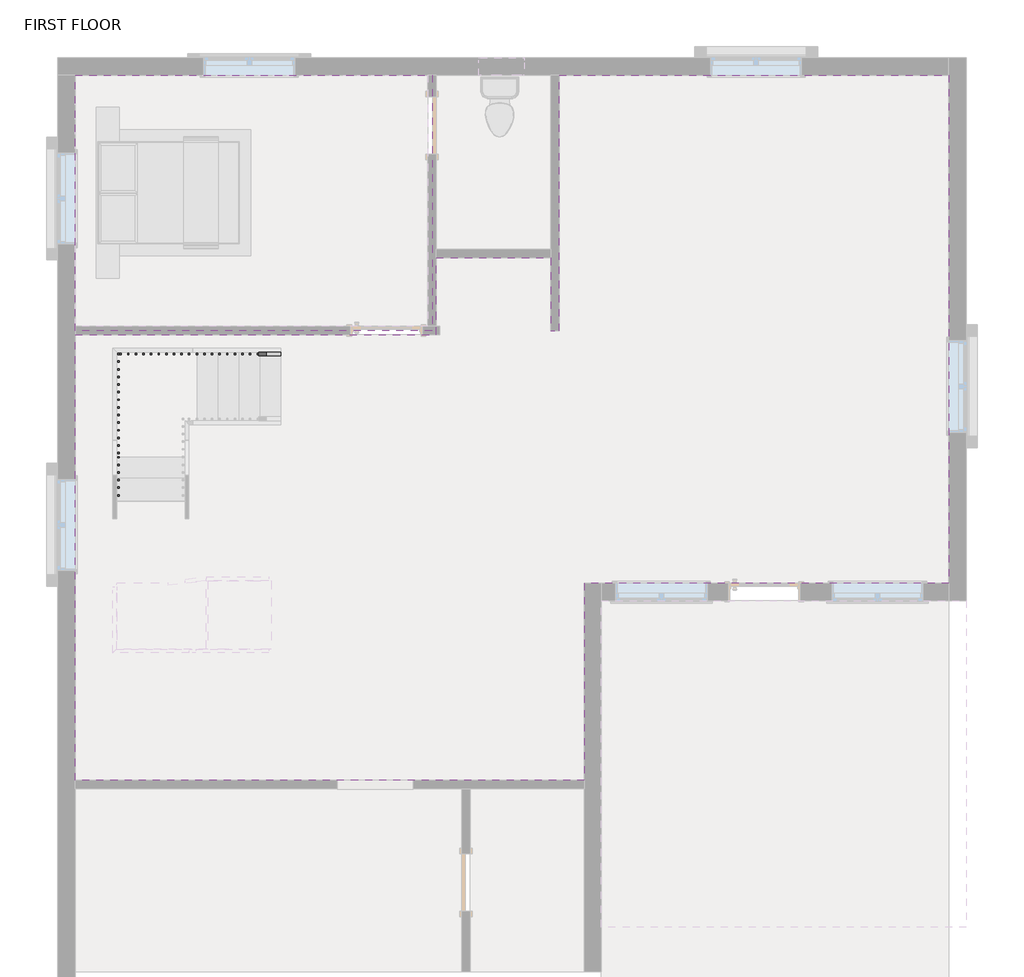
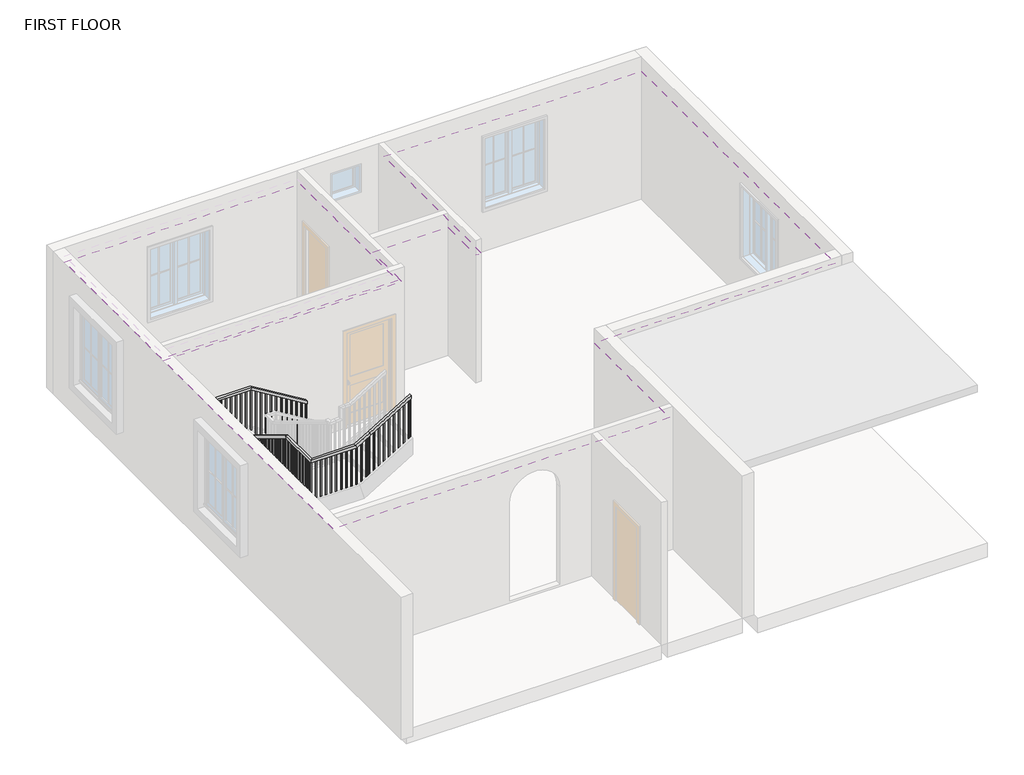
# One storey, part 2 of 4: 2 coverings, 1 railing.
"""IFC4 building model written with IfcOpenShell, lengths in millimetres."""

from ifc_helpers import new_model, si_unit, frame, origin, place, context, project, spatial, polyline, outline, extrude, faceted_brep, element, save

model = new_model("IFC4")

# Units and contexts
model_context = context("Model", 3, world=origin())
ifc_project = project(units=[si_unit("LENGTHUNIT", "METRE", prefix="MILLI")], contexts=[model_context])

# Site, building, storey
site = spatial("IfcSite", under=ifc_project)
building = spatial("IfcBuilding", under=site)
storey = spatial("IfcBuildingStorey", under=building, Name="FIRST FLOOR", Elevation=3352.8)

# Coverings
placement = place(None, origin())
element("IfcCovering", 1, ObjectType="WHITE CEILING", at=placement, inside=storey, context=model_context, shape_type="SweptSolid", body=[
    extrude(outline(polyline([(-7058.5586008, 4742.0155883), (-7058.5586008, 1332.0655883), (-11821.0586008, 1332.0655883), (-11821.0586008, 4742.0155883), (-7058.5586008, 4742.0155883)]), holes=[polyline([(-7363.3586008, 4437.2155883), (-11516.2586008, 4437.2155883), (-11516.2586008, 1636.8655883), (-7363.3586008, 1636.8655883), (-7363.3586008, 4437.2155883)])]), frame((0.0, 0.0, 6096.0), z_axis=(0.0, 0.0, 1.0), x_axis=(1.0, 0.0, 0.0)), (0.0, 0.0, 1.0), 107.95),
    extrude(outline(polyline([(-7922.1586008, 3878.4155883), (-7922.1586008, 2195.6655883), (-10957.4586008, 2195.6655883), (-10957.4586008, 3878.4155883), (-7922.1586008, 3878.4155883)]), holes=[polyline([(-7972.9586008, 3827.6155883), (-10906.6586008, 3827.6155883), (-10906.6586008, 2246.4655883), (-7972.9586008, 2246.4655883), (-7972.9586008, 3827.6155883)])]), frame((0.0, 0.0, 6096.0), z_axis=(0.0, 0.0, 1.0), x_axis=(1.0, 0.0, 0.0)), (0.0, 0.0, 1.0), 107.95),
    extrude(outline(polyline([(-8023.7586008, 3776.8155883), (-8023.7586008, 2297.2655883), (-10855.8586008, 2297.2655883), (-10855.8586008, 3776.8155883), (-8023.7586008, 3776.8155883)]), holes=[polyline([(-8074.5586008, 3726.0155883), (-10805.0586008, 3726.0155883), (-10805.0586008, 2348.0655883), (-8074.5586008, 2348.0655883), (-8074.5586008, 3726.0155883)])]), frame((0.0, 0.0, 6096.0), z_axis=(0.0, 0.0, 1.0), x_axis=(1.0, 0.0, 0.0)), (0.0, 0.0, 1.0), 107.95),
    extrude(outline(polyline([(-8125.3586008, 3675.2155883), (-8125.3586008, 2398.8655883), (-10754.2586008, 2398.8655883), (-10754.2586008, 3675.2155883), (-8125.3586008, 3675.2155883)]), holes=[polyline([(-8176.1586008, 3624.4155883), (-10703.4586008, 3624.4155883), (-10703.4586008, 2449.6655883), (-8176.1586008, 2449.6655883), (-8176.1586008, 3624.4155883)])]), frame((0.0, 0.0, 6096.0), z_axis=(0.0, 0.0, 1.0), x_axis=(1.0, 0.0, 0.0)), (0.0, 0.0, 1.0), 107.95),
    extrude(outline(polyline([(-8226.9586008, 3573.6155883), (-8226.9586008, 2500.4655883), (-10652.6586008, 2500.4655883), (-10652.6586008, 3573.6155883), (-8226.9586008, 3573.6155883)]), holes=[polyline([(-8277.7586008, 3522.8155883), (-10601.8586008, 3522.8155883), (-10601.8586008, 2551.2655883), (-8277.7586008, 2551.2655883), (-8277.7586008, 3522.8155883)])]), frame((0.0, 0.0, 6096.0), z_axis=(0.0, 0.0, 1.0), x_axis=(1.0, 0.0, 0.0)), (0.0, 0.0, 1.0), 107.95),
    extrude(outline(polyline([(-8421.7314219, 3141.5453687), (-8421.7314219, 3039.9453687), (-10326.7314219, 3039.9453687), (-10326.7314219, 3141.5453687), (-8421.7314219, 3141.5453687)])), frame((0.0, 0.0, 6096.0), z_axis=(0.0, 0.0, 1.0), x_axis=(1.0, 0.0, 0.0)), (0.0, 0.0, 1.0), 107.95),
    extrude(outline(polyline([(-8421.7314219, 3427.2953687), (-8421.7314219, 3325.6953687), (-10326.7314219, 3325.6953687), (-10326.7314219, 3427.2953687), (-8421.7314219, 3427.2953687)])), frame((0.0, 0.0, 6096.0), z_axis=(0.0, 0.0, 1.0), x_axis=(1.0, 0.0, 0.0)), (0.0, 0.0, 1.0), 107.95),
    extrude(outline(polyline([(-8421.7314219, 2798.6453687), (-8421.7314219, 2697.0453687), (-10326.7314219, 2697.0453687), (-10326.7314219, 2798.6453687), (-8421.7314219, 2798.6453687)])), frame((0.0, 0.0, 6096.0), z_axis=(0.0, 0.0, 1.0), x_axis=(1.0, 0.0, 0.0)), (0.0, 0.0, 1.0), 107.95),
])
element("IfcCovering", 2, ObjectType="WHITE CEILING", at=placement, inside=storey, context=model_context, shape_type="SweptSolid", body=[
    extrude(outline(polyline([(-5363.1086008, 1332.0655883), (-5363.1086008, 4742.0155883), (-162.4586008, 4742.0155883), (-162.4586008, -2039.7844117), (-5026.5586008, -2039.7844117), (-5026.5586008, -4668.6844117), (-11821.0586008, -4668.6844117), (-11821.0586008, 1274.9155883), (-7001.4086008, 1274.9155883), (-7001.4086008, 2303.6155883), (-5477.4086008, 2303.6155883), (-5477.4086008, 1332.0655883), (-5363.1086008, 1332.0655883)]), holes=[polyline([(-9204.4022729, -2001.6844117), (-9236.1522729, -2001.6844117), (-9236.1522729, -1950.8844117), (-10074.3522729, -1950.8844117), (-10302.9522729, -1976.3421011), (-10302.9522729, -132.1404207), (-10302.9522729, 79.9115003), (-9079.7156858, 79.9115003), (-9079.7156858, 130.7115003), (-9079.7156858, 181.5115003), (-9079.7156858, 1045.1115003), (-9079.7156858, 1095.9115003), (-11318.9522729, 1095.9115003), (-11318.9522729, -2966.8844117), (-10213.4567611, -2966.8844117), (-9236.1522729, -2966.8844117), (-9236.1522729, -2916.0844117), (-9204.4022729, -2916.0844117), (-9204.4022729, -2001.6844117)])]), frame((0.0, 0.0, 6096.0), z_axis=(0.0, 0.0, 1.0), x_axis=(1.0, 0.0, 0.0)), (0.0, 0.0, 1.0), 107.95),
])

# Railing
element("IfcRailing", 3, ObjectType="Handrail - Rectangular", at=placement, inside=storey, context=model_context, shape_type="SolidModel", body=[
    faceted_brep([(-9079.7156858, 994.3115003, 4436.5333333), (-9079.7156858, 994.3115003, 4377.1318731), (-9079.7156858, 1045.1115003, 4377.1318731), (-9079.7156858, 1045.1115003, 4436.5333333), (-10197.3156858, 994.3115003, 5113.8666667), (-10211.5080953, 994.3115003, 5063.0666667), (-10211.5080953, 1045.1115003, 5063.0666667), (-10197.3156858, 1045.1115003, 5113.8666667), (-11217.3522729, 994.3115003, 5113.8666667), (-11217.3522729, 994.3115003, 5063.0666667), (-11268.1522729, 1045.1115003, 5063.0666667), (-11268.1522729, 1045.1115003, 5113.8666667), (-11217.3522729, -76.9993654, 5113.8666667), (-11217.3522729, -91.1917748, 5063.0666667), (-11268.1522729, -91.1917748, 5063.0666667), (-11268.1522729, -76.9993654, 5113.8666667), (-11217.3522729, -356.3993654, 5283.2), (-11217.3522729, -382.7290926, 5239.7559502), (-11268.1522729, -382.7290926, 5239.7559502), (-11268.1522729, -356.3993654, 5283.2), (-11217.3522729, -2032.7993654, 6299.2), (-11217.3522729, -2046.9917748, 6248.4), (-11268.1522729, -2046.9917748, 6248.4), (-11268.1522729, -2032.7993654, 6299.2), (-11217.3522729, -2865.2844117, 6299.2), (-11217.3522729, -2865.2844117, 6248.4), (-11268.1522729, -2916.0844117, 6248.4), (-11268.1522729, -2916.0844117, 6299.2), (-10353.7522729, -2865.2844117, 6299.2), (-10339.5598635, -2865.2844117, 6248.4), (-10339.5598635, -2916.0844117, 6248.4), (-10353.7522729, -2916.0844117, 6299.2), (-10074.3522729, -2865.2844117, 6468.5333333), (-10048.0225457, -2865.2844117, 6425.0892835), (-10048.0225457, -2916.0844117, 6425.0892835), (-10074.3522729, -2916.0844117, 6468.5333333), (-9236.1522729, -2865.2844117, 6976.5333333), (-9236.1522729, -2916.0844117, 6976.5333333), (-9236.1522729, -2916.0844117, 6917.1318731), (-9236.1522729, -2865.2844117, 6917.1318731)], [[[0, 1, 2, 3]], [[1, 0, 4, 5]], [[2, 1, 5, 6]], [[3, 2, 6, 7]], [[0, 3, 7, 4]], [[5, 4, 8, 9]], [[6, 5, 9, 10]], [[7, 6, 10, 11]], [[4, 7, 11, 8]], [[9, 8, 12, 13]], [[10, 9, 13, 14]], [[11, 10, 14, 15]], [[8, 11, 15, 12]], [[13, 12, 16, 17]], [[14, 13, 17, 18]], [[15, 14, 18, 19]], [[12, 15, 19, 16]], [[17, 16, 20, 21]], [[18, 17, 21, 22]], [[19, 18, 22, 23]], [[16, 19, 23, 20]], [[21, 20, 24, 25]], [[22, 21, 25, 26]], [[23, 22, 26, 27]], [[20, 23, 27, 24]], [[25, 24, 28, 29]], [[26, 25, 29, 30]], [[27, 26, 30, 31]], [[24, 27, 31, 28]], [[29, 28, 32, 33]], [[30, 29, 33, 34]], [[31, 30, 34, 35]], [[28, 31, 35, 32]], [[36, 37, 38, 39]], [[33, 32, 36, 39]], [[34, 33, 39, 38]], [[35, 34, 38, 37]], [[32, 35, 37, 36]]]),
    extrude(outline(polyline([(6907.510661, -9252.0272729), (6895.9652064, -9271.0772729), (5892.8, -9271.0772729), (5892.8, -9252.0272729), (6907.510661, -9252.0272729)])), frame((0.0, -2900.2094117, 0.0), z_axis=(0.0, 1.0, 0.0), x_axis=(0.0, 0.0, 1.0)), (0.0, 0.0, 1.0), 19.05),
    extrude(outline(polyline([(6845.9349034, -9353.6272729), (6834.3894488, -9372.6772729), (5892.8, -9372.6772729), (5892.8, -9353.6272729), (6845.9349034, -9353.6272729)])), frame((0.0, -2900.2094117, 0.0), z_axis=(0.0, 1.0, 0.0), x_axis=(0.0, 0.0, 1.0)), (0.0, 0.0, 1.0), 19.05),
    extrude(outline(polyline([(6784.3591458, -9455.2272729), (6772.8136913, -9474.2772729), (5892.8, -9474.2772729), (5892.8, -9455.2272729), (6784.3591458, -9455.2272729)])), frame((0.0, -2900.2094117, 0.0), z_axis=(0.0, 1.0, 0.0), x_axis=(0.0, 0.0, 1.0)), (0.0, 0.0, 1.0), 19.05),
    extrude(outline(polyline([(6722.7833882, -9556.8272729), (6711.2379337, -9575.8772729), (5723.4666667, -9575.8772729), (5723.4666667, -9556.8272729), (6722.7833882, -9556.8272729)])), frame((0.0, -2900.2094117, 0.0), z_axis=(0.0, 1.0, 0.0), x_axis=(0.0, 0.0, 1.0)), (0.0, 0.0, 1.0), 19.05),
    extrude(outline(polyline([(6661.2076307, -9658.4272729), (6649.6621761, -9677.4772729), (5723.4666667, -9677.4772729), (5723.4666667, -9658.4272729), (6661.2076307, -9658.4272729)])), frame((0.0, -2900.2094117, 0.0), z_axis=(0.0, 1.0, 0.0), x_axis=(0.0, 0.0, 1.0)), (0.0, 0.0, 1.0), 19.05),
    extrude(outline(polyline([(6599.6318731, -9760.0272729), (6588.0864185, -9779.0772729), (5723.4666667, -9779.0772729), (5723.4666667, -9760.0272729), (6599.6318731, -9760.0272729)])), frame((0.0, -2900.2094117, 0.0), z_axis=(0.0, 1.0, 0.0), x_axis=(0.0, 0.0, 1.0)), (0.0, 0.0, 1.0), 19.05),
    extrude(outline(polyline([(6538.0561155, -9861.6272729), (6526.510661, -9880.6772729), (5554.1333333, -9880.6772729), (5554.1333333, -9861.6272729), (6538.0561155, -9861.6272729)])), frame((0.0, -2900.2094117, 0.0), z_axis=(0.0, 1.0, 0.0), x_axis=(0.0, 0.0, 1.0)), (0.0, 0.0, 1.0), 19.05),
    extrude(outline(polyline([(6476.4803579, -9963.2272729), (6464.9349034, -9982.2772729), (5554.1333333, -9982.2772729), (5554.1333333, -9963.2272729), (6476.4803579, -9963.2272729)])), frame((0.0, -2900.2094117, 0.0), z_axis=(0.0, 1.0, 0.0), x_axis=(0.0, 0.0, 1.0)), (0.0, 0.0, 1.0), 19.05),
    extrude(outline(polyline([(6384.1167216, -10115.6272729), (6372.571267, -10134.6772729), (5384.8, -10134.6772729), (5384.8, -10115.6272729), (6384.1167216, -10115.6272729)])), frame((0.0, -2900.2094117, 0.0), z_axis=(0.0, 1.0, 0.0), x_axis=(0.0, 0.0, 1.0)), (0.0, 0.0, 1.0), 19.05),
    extrude(outline(polyline([(6322.540964, -10217.2272729), (6310.9955094, -10236.2772729), (5384.8, -10236.2772729), (5384.8, -10217.2272729), (6322.540964, -10217.2272729)])), frame((0.0, -2900.2094117, 0.0), z_axis=(0.0, 1.0, 0.0), x_axis=(0.0, 0.0, 1.0)), (0.0, 0.0, 1.0), 19.05),
    extrude(outline(polyline([(6260.9652064, -10318.8272729), (6249.4197519, -10337.8772729), (5384.8, -10337.8772729), (5384.8, -10318.8272729), (6260.9652064, -10318.8272729)])), frame((0.0, -2900.2094117, 0.0), z_axis=(0.0, 1.0, 0.0), x_axis=(0.0, 0.0, 1.0)), (0.0, 0.0, 1.0), 19.05),
    extrude(outline(polyline([(-10439.4772729, -2900.2094117), (-10439.4772729, -2881.1594117), (-10420.4272729, -2881.1594117), (-10420.4272729, -2900.2094117), (-10439.4772729, -2900.2094117)])), frame((0.0, 0.0, 5384.8), z_axis=(0.0, 0.0, 1.0), x_axis=(1.0, 0.0, 0.0)), (0.0, 0.0, 1.0), 863.6),
    extrude(outline(polyline([(-10541.0772729, -2900.2094117), (-10541.0772729, -2881.1594117), (-10522.0272729, -2881.1594117), (-10522.0272729, -2900.2094117), (-10541.0772729, -2900.2094117)])), frame((0.0, 0.0, 5384.8), z_axis=(0.0, 0.0, 1.0), x_axis=(1.0, 0.0, 0.0)), (0.0, 0.0, 1.0), 863.6),
    extrude(outline(polyline([(-10642.6772729, -2900.2094117), (-10642.6772729, -2881.1594117), (-10623.6272729, -2881.1594117), (-10623.6272729, -2900.2094117), (-10642.6772729, -2900.2094117)])), frame((0.0, 0.0, 5384.8), z_axis=(0.0, 0.0, 1.0), x_axis=(1.0, 0.0, 0.0)), (0.0, 0.0, 1.0), 863.6),
    extrude(outline(polyline([(-10744.2772729, -2900.2094117), (-10744.2772729, -2881.1594117), (-10725.2272729, -2881.1594117), (-10725.2272729, -2900.2094117), (-10744.2772729, -2900.2094117)])), frame((0.0, 0.0, 5384.8), z_axis=(0.0, 0.0, 1.0), x_axis=(1.0, 0.0, 0.0)), (0.0, 0.0, 1.0), 863.6),
    extrude(outline(polyline([(-10845.8772729, -2900.2094117), (-10845.8772729, -2881.1594117), (-10826.8272729, -2881.1594117), (-10826.8272729, -2900.2094117), (-10845.8772729, -2900.2094117)])), frame((0.0, 0.0, 5384.8), z_axis=(0.0, 0.0, 1.0), x_axis=(1.0, 0.0, 0.0)), (0.0, 0.0, 1.0), 863.6),
    extrude(outline(polyline([(-10947.4772729, -2900.2094117), (-10947.4772729, -2881.1594117), (-10928.4272729, -2881.1594117), (-10928.4272729, -2900.2094117), (-10947.4772729, -2900.2094117)])), frame((0.0, 0.0, 5384.8), z_axis=(0.0, 0.0, 1.0), x_axis=(1.0, 0.0, 0.0)), (0.0, 0.0, 1.0), 863.6),
    extrude(outline(polyline([(-11049.0772729, -2900.2094117), (-11049.0772729, -2881.1594117), (-11030.0272729, -2881.1594117), (-11030.0272729, -2900.2094117), (-11049.0772729, -2900.2094117)])), frame((0.0, 0.0, 5384.8), z_axis=(0.0, 0.0, 1.0), x_axis=(1.0, 0.0, 0.0)), (0.0, 0.0, 1.0), 863.6),
    extrude(outline(polyline([(-11150.6772729, -2900.2094117), (-11150.6772729, -2881.1594117), (-11131.6272729, -2881.1594117), (-11131.6272729, -2900.2094117), (-11150.6772729, -2900.2094117)])), frame((0.0, 0.0, 5384.8), z_axis=(0.0, 0.0, 1.0), x_axis=(1.0, 0.0, 0.0)), (0.0, 0.0, 1.0), 863.6),
    extrude(outline(polyline([(-11252.2772729, -2836.0743654), (-11233.2272729, -2836.0743654), (-11233.2272729, -2855.1243654), (-11252.2772729, -2855.1243654), (-11252.2772729, -2836.0743654)])), frame((0.0, 0.0, 5384.8), z_axis=(0.0, 0.0, 1.0), x_axis=(1.0, 0.0, 0.0)), (0.0, 0.0, 1.0), 863.6),
    extrude(outline(polyline([(-11252.2772729, -2734.4743654), (-11233.2272729, -2734.4743654), (-11233.2272729, -2753.5243654), (-11252.2772729, -2753.5243654), (-11252.2772729, -2734.4743654)])), frame((0.0, 0.0, 5384.8), z_axis=(0.0, 0.0, 1.0), x_axis=(1.0, 0.0, 0.0)), (0.0, 0.0, 1.0), 863.6),
    extrude(outline(polyline([(-11252.2772729, -2632.8743654), (-11233.2272729, -2632.8743654), (-11233.2272729, -2651.9243654), (-11252.2772729, -2651.9243654), (-11252.2772729, -2632.8743654)])), frame((0.0, 0.0, 5384.8), z_axis=(0.0, 0.0, 1.0), x_axis=(1.0, 0.0, 0.0)), (0.0, 0.0, 1.0), 863.6),
    extrude(outline(polyline([(-11252.2772729, -2531.2743654), (-11233.2272729, -2531.2743654), (-11233.2272729, -2550.3243654), (-11252.2772729, -2550.3243654), (-11252.2772729, -2531.2743654)])), frame((0.0, 0.0, 5384.8), z_axis=(0.0, 0.0, 1.0), x_axis=(1.0, 0.0, 0.0)), (0.0, 0.0, 1.0), 863.6),
    extrude(outline(polyline([(-11252.2772729, -2429.6743654), (-11233.2272729, -2429.6743654), (-11233.2272729, -2448.7243654), (-11252.2772729, -2448.7243654), (-11252.2772729, -2429.6743654)])), frame((0.0, 0.0, 5384.8), z_axis=(0.0, 0.0, 1.0), x_axis=(1.0, 0.0, 0.0)), (0.0, 0.0, 1.0), 863.6),
    extrude(outline(polyline([(-11252.2772729, -2328.0743654), (-11233.2272729, -2328.0743654), (-11233.2272729, -2347.1243654), (-11252.2772729, -2347.1243654), (-11252.2772729, -2328.0743654)])), frame((0.0, 0.0, 5384.8), z_axis=(0.0, 0.0, 1.0), x_axis=(1.0, 0.0, 0.0)), (0.0, 0.0, 1.0), 863.6),
    extrude(outline(polyline([(-11252.2772729, -2226.4743654), (-11233.2272729, -2226.4743654), (-11233.2272729, -2245.5243654), (-11252.2772729, -2245.5243654), (-11252.2772729, -2226.4743654)])), frame((0.0, 0.0, 5384.8), z_axis=(0.0, 0.0, 1.0), x_axis=(1.0, 0.0, 0.0)), (0.0, 0.0, 1.0), 863.6),
    extrude(outline(polyline([(-11252.2772729, -2124.8743654), (-11233.2272729, -2124.8743654), (-11233.2272729, -2143.9243654), (-11252.2772729, -2143.9243654), (-11252.2772729, -2124.8743654)])), frame((0.0, 0.0, 5384.8), z_axis=(0.0, 0.0, 1.0), x_axis=(1.0, 0.0, 0.0)), (0.0, 0.0, 1.0), 863.6),
    extrude(outline(polyline([(-1991.5243654, 6214.7833882), (-1972.4743654, 6203.2379337), (-1972.4743654, 5215.4666667), (-1991.5243654, 5215.4666667), (-1991.5243654, 6214.7833882)])), frame((-11252.2772729, 0.0, 0.0), z_axis=(1.0, 0.0, 0.0), x_axis=(0.0, 1.0, 0.0)), (0.0, 0.0, 1.0), 19.05),
    extrude(outline(polyline([(-1889.9243654, 6153.2076307), (-1870.8743654, 6141.6621761), (-1870.8743654, 5215.4666667), (-1889.9243654, 5215.4666667), (-1889.9243654, 6153.2076307)])), frame((-11252.2772729, 0.0, 0.0), z_axis=(1.0, 0.0, 0.0), x_axis=(0.0, 1.0, 0.0)), (0.0, 0.0, 1.0), 19.05),
    extrude(outline(polyline([(-1788.3243654, 6091.6318731), (-1769.2743654, 6080.0864185), (-1769.2743654, 5215.4666667), (-1788.3243654, 5215.4666667), (-1788.3243654, 6091.6318731)])), frame((-11252.2772729, 0.0, 0.0), z_axis=(1.0, 0.0, 0.0), x_axis=(0.0, 1.0, 0.0)), (0.0, 0.0, 1.0), 19.05),
    extrude(outline(polyline([(-1686.7243654, 6030.0561155), (-1667.6743654, 6018.510661), (-1667.6743654, 5046.1333333), (-1686.7243654, 5046.1333333), (-1686.7243654, 6030.0561155)])), frame((-11252.2772729, 0.0, 0.0), z_axis=(1.0, 0.0, 0.0), x_axis=(0.0, 1.0, 0.0)), (0.0, 0.0, 1.0), 19.05),
    extrude(outline(polyline([(-1585.1243654, 5968.4803579), (-1566.0743654, 5956.9349034), (-1566.0743654, 5046.1333333), (-1585.1243654, 5046.1333333), (-1585.1243654, 5968.4803579)])), frame((-11252.2772729, 0.0, 0.0), z_axis=(1.0, 0.0, 0.0), x_axis=(0.0, 1.0, 0.0)), (0.0, 0.0, 1.0), 19.05),
    extrude(outline(polyline([(-1483.5243654, 5906.9046004), (-1464.4743654, 5895.3591458), (-1464.4743654, 5046.1333333), (-1483.5243654, 5046.1333333), (-1483.5243654, 5906.9046004)])), frame((-11252.2772729, 0.0, 0.0), z_axis=(1.0, 0.0, 0.0), x_axis=(0.0, 1.0, 0.0)), (0.0, 0.0, 1.0), 19.05),
    extrude(outline(polyline([(-1381.9243654, 5845.3288428), (-1362.8743654, 5833.7833882), (-1362.8743654, 4876.8), (-1381.9243654, 4876.8), (-1381.9243654, 5845.3288428)])), frame((-11252.2772729, 0.0, 0.0), z_axis=(1.0, 0.0, 0.0), x_axis=(0.0, 1.0, 0.0)), (0.0, 0.0, 1.0), 19.05),
    extrude(outline(polyline([(-1280.3243654, 5783.7530852), (-1261.2743654, 5772.2076307), (-1261.2743654, 4876.8), (-1280.3243654, 4876.8), (-1280.3243654, 5783.7530852)])), frame((-11252.2772729, 0.0, 0.0), z_axis=(1.0, 0.0, 0.0), x_axis=(0.0, 1.0, 0.0)), (0.0, 0.0, 1.0), 19.05),
    extrude(outline(polyline([(-1178.7243654, 5722.1773276), (-1159.6743654, 5710.6318731), (-1159.6743654, 4707.4666667), (-1178.7243654, 4707.4666667), (-1178.7243654, 5722.1773276)])), frame((-11252.2772729, 0.0, 0.0), z_axis=(1.0, 0.0, 0.0), x_axis=(0.0, 1.0, 0.0)), (0.0, 0.0, 1.0), 19.05),
    extrude(outline(polyline([(-1077.1243654, 5660.60157), (-1058.0743654, 5649.0561155), (-1058.0743654, 4707.4666667), (-1077.1243654, 4707.4666667), (-1077.1243654, 5660.60157)])), frame((-11252.2772729, 0.0, 0.0), z_axis=(1.0, 0.0, 0.0), x_axis=(0.0, 1.0, 0.0)), (0.0, 0.0, 1.0), 19.05),
    extrude(outline(polyline([(-975.5243654, 5599.0258125), (-956.4743654, 5587.4803579), (-956.4743654, 4707.4666667), (-975.5243654, 4707.4666667), (-975.5243654, 5599.0258125)])), frame((-11252.2772729, 0.0, 0.0), z_axis=(1.0, 0.0, 0.0), x_axis=(0.0, 1.0, 0.0)), (0.0, 0.0, 1.0), 19.05),
    extrude(outline(polyline([(-873.9243654, 5537.4500549), (-854.8743654, 5525.9046004), (-854.8743654, 4538.1333333), (-873.9243654, 4538.1333333), (-873.9243654, 5537.4500549)])), frame((-11252.2772729, 0.0, 0.0), z_axis=(1.0, 0.0, 0.0), x_axis=(0.0, 1.0, 0.0)), (0.0, 0.0, 1.0), 19.05),
    extrude(outline(polyline([(-772.3243654, 5475.8742973), (-753.2743654, 5464.3288428), (-753.2743654, 4538.1333333), (-772.3243654, 4538.1333333), (-772.3243654, 5475.8742973)])), frame((-11252.2772729, 0.0, 0.0), z_axis=(1.0, 0.0, 0.0), x_axis=(0.0, 1.0, 0.0)), (0.0, 0.0, 1.0), 19.05),
    extrude(outline(polyline([(-670.7243654, 5414.2985397), (-651.6743654, 5402.7530852), (-651.6743654, 4538.1333333), (-670.7243654, 4538.1333333), (-670.7243654, 5414.2985397)])), frame((-11252.2772729, 0.0, 0.0), z_axis=(1.0, 0.0, 0.0), x_axis=(0.0, 1.0, 0.0)), (0.0, 0.0, 1.0), 19.05),
    extrude(outline(polyline([(-569.1243654, 5352.7227822), (-550.0743654, 5341.1773276), (-550.0743654, 4368.8), (-569.1243654, 4368.8), (-569.1243654, 5352.7227822)])), frame((-11252.2772729, 0.0, 0.0), z_axis=(1.0, 0.0, 0.0), x_axis=(0.0, 1.0, 0.0)), (0.0, 0.0, 1.0), 19.05),
    extrude(outline(polyline([(-467.5243654, 5291.1470246), (-448.4743654, 5279.60157), (-448.4743654, 4368.8), (-467.5243654, 4368.8), (-467.5243654, 5291.1470246)])), frame((-11252.2772729, 0.0, 0.0), z_axis=(1.0, 0.0, 0.0), x_axis=(0.0, 1.0, 0.0)), (0.0, 0.0, 1.0), 19.05),
    extrude(outline(polyline([(-310.6134997, 5196.0495303), (-291.5634997, 5184.5040757), (-291.5634997, 4199.4666667), (-310.6134997, 4199.4666667), (-310.6134997, 5196.0495303)])), frame((-11252.2772729, 0.0, 0.0), z_axis=(1.0, 0.0, 0.0), x_axis=(0.0, 1.0, 0.0)), (0.0, 0.0, 1.0), 19.05),
    extrude(outline(polyline([(-209.0134997, 5134.4737727), (-189.9634997, 5122.9283181), (-189.9634997, 4199.4666667), (-209.0134997, 4199.4666667), (-209.0134997, 5134.4737727)])), frame((-11252.2772729, 0.0, 0.0), z_axis=(1.0, 0.0, 0.0), x_axis=(0.0, 1.0, 0.0)), (0.0, 0.0, 1.0), 19.05),
    extrude(outline(polyline([(-107.4134997, 5072.8980151), (-88.3634997, 5061.3525606), (-88.3634997, 4199.4666667), (-107.4134997, 4199.4666667), (-107.4134997, 5072.8980151)])), frame((-11252.2772729, 0.0, 0.0), z_axis=(1.0, 0.0, 0.0), x_axis=(0.0, 1.0, 0.0)), (0.0, 0.0, 1.0), 19.05),
    extrude(outline(polyline([(-11252.2772729, 13.2365003), (-11233.2272729, 13.2365003), (-11233.2272729, -5.8134997), (-11252.2772729, -5.8134997), (-11252.2772729, 13.2365003)])), frame((0.0, 0.0, 4199.4666667), z_axis=(0.0, 0.0, 1.0), x_axis=(1.0, 0.0, 0.0)), (0.0, 0.0, 1.0), 863.6),
    extrude(outline(polyline([(-11252.2772729, 114.8365003), (-11233.2272729, 114.8365003), (-11233.2272729, 95.7865003), (-11252.2772729, 95.7865003), (-11252.2772729, 114.8365003)])), frame((0.0, 0.0, 4199.4666667), z_axis=(0.0, 0.0, 1.0), x_axis=(1.0, 0.0, 0.0)), (0.0, 0.0, 1.0), 863.6),
    extrude(outline(polyline([(-11252.2772729, 216.4365003), (-11233.2272729, 216.4365003), (-11233.2272729, 197.3865003), (-11252.2772729, 197.3865003), (-11252.2772729, 216.4365003)])), frame((0.0, 0.0, 4199.4666667), z_axis=(0.0, 0.0, 1.0), x_axis=(1.0, 0.0, 0.0)), (0.0, 0.0, 1.0), 863.6),
    extrude(outline(polyline([(-11252.2772729, 318.0365003), (-11233.2272729, 318.0365003), (-11233.2272729, 298.9865003), (-11252.2772729, 298.9865003), (-11252.2772729, 318.0365003)])), frame((0.0, 0.0, 4199.4666667), z_axis=(0.0, 0.0, 1.0), x_axis=(1.0, 0.0, 0.0)), (0.0, 0.0, 1.0), 863.6),
    extrude(outline(polyline([(-11252.2772729, 419.6365003), (-11233.2272729, 419.6365003), (-11233.2272729, 400.5865003), (-11252.2772729, 400.5865003), (-11252.2772729, 419.6365003)])), frame((0.0, 0.0, 4199.4666667), z_axis=(0.0, 0.0, 1.0), x_axis=(1.0, 0.0, 0.0)), (0.0, 0.0, 1.0), 863.6),
    extrude(outline(polyline([(-11252.2772729, 521.2365003), (-11233.2272729, 521.2365003), (-11233.2272729, 502.1865003), (-11252.2772729, 502.1865003), (-11252.2772729, 521.2365003)])), frame((0.0, 0.0, 4199.4666667), z_axis=(0.0, 0.0, 1.0), x_axis=(1.0, 0.0, 0.0)), (0.0, 0.0, 1.0), 863.6),
    extrude(outline(polyline([(-11252.2772729, 622.8365003), (-11233.2272729, 622.8365003), (-11233.2272729, 603.7865003), (-11252.2772729, 603.7865003), (-11252.2772729, 622.8365003)])), frame((0.0, 0.0, 4199.4666667), z_axis=(0.0, 0.0, 1.0), x_axis=(1.0, 0.0, 0.0)), (0.0, 0.0, 1.0), 863.6),
    extrude(outline(polyline([(-11252.2772729, 724.4365003), (-11233.2272729, 724.4365003), (-11233.2272729, 705.3865003), (-11252.2772729, 705.3865003), (-11252.2772729, 724.4365003)])), frame((0.0, 0.0, 4199.4666667), z_axis=(0.0, 0.0, 1.0), x_axis=(1.0, 0.0, 0.0)), (0.0, 0.0, 1.0), 863.6),
    extrude(outline(polyline([(-11252.2772729, 826.0365003), (-11233.2272729, 826.0365003), (-11233.2272729, 806.9865003), (-11252.2772729, 806.9865003), (-11252.2772729, 826.0365003)])), frame((0.0, 0.0, 4199.4666667), z_axis=(0.0, 0.0, 1.0), x_axis=(1.0, 0.0, 0.0)), (0.0, 0.0, 1.0), 863.6),
    extrude(outline(polyline([(-11252.2772729, 927.6365003), (-11233.2272729, 927.6365003), (-11233.2272729, 908.5865003), (-11252.2772729, 908.5865003), (-11252.2772729, 927.6365003)])), frame((0.0, 0.0, 4199.4666667), z_axis=(0.0, 0.0, 1.0), x_axis=(1.0, 0.0, 0.0)), (0.0, 0.0, 1.0), 863.6),
    extrude(outline(polyline([(-11203.7906858, 1029.2365003), (-11203.7906858, 1010.1865003), (-11222.8406858, 1010.1865003), (-11222.8406858, 1029.2365003), (-11203.7906858, 1029.2365003)])), frame((0.0, 0.0, 4199.4666667), z_axis=(0.0, 0.0, 1.0), x_axis=(1.0, 0.0, 0.0)), (0.0, 0.0, 1.0), 863.6),
    extrude(outline(polyline([(-11102.1906858, 1029.2365003), (-11102.1906858, 1010.1865003), (-11121.2406858, 1010.1865003), (-11121.2406858, 1029.2365003), (-11102.1906858, 1029.2365003)])), frame((0.0, 0.0, 4199.4666667), z_axis=(0.0, 0.0, 1.0), x_axis=(1.0, 0.0, 0.0)), (0.0, 0.0, 1.0), 863.6),
    extrude(outline(polyline([(-11000.5906858, 1029.2365003), (-11000.5906858, 1010.1865003), (-11019.6406858, 1010.1865003), (-11019.6406858, 1029.2365003), (-11000.5906858, 1029.2365003)])), frame((0.0, 0.0, 4199.4666667), z_axis=(0.0, 0.0, 1.0), x_axis=(1.0, 0.0, 0.0)), (0.0, 0.0, 1.0), 863.6),
    extrude(outline(polyline([(-10898.9906858, 1029.2365003), (-10898.9906858, 1010.1865003), (-10918.0406858, 1010.1865003), (-10918.0406858, 1029.2365003), (-10898.9906858, 1029.2365003)])), frame((0.0, 0.0, 4199.4666667), z_axis=(0.0, 0.0, 1.0), x_axis=(1.0, 0.0, 0.0)), (0.0, 0.0, 1.0), 863.6),
    extrude(outline(polyline([(-10797.3906858, 1029.2365003), (-10797.3906858, 1010.1865003), (-10816.4406858, 1010.1865003), (-10816.4406858, 1029.2365003), (-10797.3906858, 1029.2365003)])), frame((0.0, 0.0, 4199.4666667), z_axis=(0.0, 0.0, 1.0), x_axis=(1.0, 0.0, 0.0)), (0.0, 0.0, 1.0), 863.6),
    extrude(outline(polyline([(-10695.7906858, 1029.2365003), (-10695.7906858, 1010.1865003), (-10714.8406858, 1010.1865003), (-10714.8406858, 1029.2365003), (-10695.7906858, 1029.2365003)])), frame((0.0, 0.0, 4199.4666667), z_axis=(0.0, 0.0, 1.0), x_axis=(1.0, 0.0, 0.0)), (0.0, 0.0, 1.0), 863.6),
    extrude(outline(polyline([(-10594.1906858, 1029.2365003), (-10594.1906858, 1010.1865003), (-10613.2406858, 1010.1865003), (-10613.2406858, 1029.2365003), (-10594.1906858, 1029.2365003)])), frame((0.0, 0.0, 4199.4666667), z_axis=(0.0, 0.0, 1.0), x_axis=(1.0, 0.0, 0.0)), (0.0, 0.0, 1.0), 863.6),
    extrude(outline(polyline([(-10492.5906858, 1029.2365003), (-10492.5906858, 1010.1865003), (-10511.6406858, 1010.1865003), (-10511.6406858, 1029.2365003), (-10492.5906858, 1029.2365003)])), frame((0.0, 0.0, 4199.4666667), z_axis=(0.0, 0.0, 1.0), x_axis=(1.0, 0.0, 0.0)), (0.0, 0.0, 1.0), 863.6),
    extrude(outline(polyline([(-10390.9906858, 1029.2365003), (-10390.9906858, 1010.1865003), (-10410.0406858, 1010.1865003), (-10410.0406858, 1029.2365003), (-10390.9906858, 1029.2365003)])), frame((0.0, 0.0, 4199.4666667), z_axis=(0.0, 0.0, 1.0), x_axis=(1.0, 0.0, 0.0)), (0.0, 0.0, 1.0), 863.6),
    extrude(outline(polyline([(-10289.3906858, 1029.2365003), (-10289.3906858, 1010.1865003), (-10308.4406858, 1010.1865003), (-10308.4406858, 1029.2365003), (-10289.3906858, 1029.2365003)])), frame((0.0, 0.0, 4199.4666667), z_axis=(0.0, 0.0, 1.0), x_axis=(1.0, 0.0, 0.0)), (0.0, 0.0, 1.0), 863.6),
    extrude(outline(polyline([(4987.1167216, -10086.1906858), (4998.6621761, -10105.2406858), (4030.1333333, -10105.2406858), (4030.1333333, -10086.1906858), (4987.1167216, -10086.1906858)])), frame((0.0, 1010.1865003, 0.0), z_axis=(0.0, 1.0, 0.0), x_axis=(0.0, 0.0, 1.0)), (0.0, 0.0, 1.0), 19.05),
    extrude(outline(polyline([(4925.540964, -9984.5906858), (4937.0864185, -10003.6406858), (4030.1333333, -10003.6406858), (4030.1333333, -9984.5906858), (4925.540964, -9984.5906858)])), frame((0.0, 1010.1865003, 0.0), z_axis=(0.0, 1.0, 0.0), x_axis=(0.0, 0.0, 1.0)), (0.0, 0.0, 1.0), 19.05),
    extrude(outline(polyline([(4863.9652064, -9882.9906858), (4875.510661, -9902.0406858), (3860.8, -9902.0406858), (3860.8, -9882.9906858), (4863.9652064, -9882.9906858)])), frame((0.0, 1010.1865003, 0.0), z_axis=(0.0, 1.0, 0.0), x_axis=(0.0, 0.0, 1.0)), (0.0, 0.0, 1.0), 19.05),
    extrude(outline(polyline([(4802.3894488, -9781.3906858), (4813.9349034, -9800.4406858), (3860.8, -9800.4406858), (3860.8, -9781.3906858), (4802.3894488, -9781.3906858)])), frame((0.0, 1010.1865003, 0.0), z_axis=(0.0, 1.0, 0.0), x_axis=(0.0, 0.0, 1.0)), (0.0, 0.0, 1.0), 19.05),
    extrude(outline(polyline([(4740.8136913, -9679.7906858), (4752.3591458, -9698.8406858), (3860.8, -9698.8406858), (3860.8, -9679.7906858), (4740.8136913, -9679.7906858)])), frame((0.0, 1010.1865003, 0.0), z_axis=(0.0, 1.0, 0.0), x_axis=(0.0, 0.0, 1.0)), (0.0, 0.0, 1.0), 19.05),
    extrude(outline(polyline([(4679.2379337, -9578.1906858), (4690.7833882, -9597.2406858), (3691.4666667, -9597.2406858), (3691.4666667, -9578.1906858), (4679.2379337, -9578.1906858)])), frame((0.0, 1010.1865003, 0.0), z_axis=(0.0, 1.0, 0.0), x_axis=(0.0, 0.0, 1.0)), (0.0, 0.0, 1.0), 19.05),
    extrude(outline(polyline([(4617.6621761, -9476.5906858), (4629.2076307, -9495.6406858), (3691.4666667, -9495.6406858), (3691.4666667, -9476.5906858), (4617.6621761, -9476.5906858)])), frame((0.0, 1010.1865003, 0.0), z_axis=(0.0, 1.0, 0.0), x_axis=(0.0, 0.0, 1.0)), (0.0, 0.0, 1.0), 19.05),
    extrude(outline(polyline([(4556.0864185, -9374.9906858), (4567.6318731, -9394.0406858), (3691.4666667, -9394.0406858), (3691.4666667, -9374.9906858), (4556.0864185, -9374.9906858)])), frame((0.0, 1010.1865003, 0.0), z_axis=(0.0, 1.0, 0.0), x_axis=(0.0, 0.0, 1.0)), (0.0, 0.0, 1.0), 19.05),
    extrude(outline(polyline([(4494.510661, -9273.3906858), (4506.0561155, -9292.4406858), (3522.1333333, -9292.4406858), (3522.1333333, -9273.3906858), (4494.510661, -9273.3906858)])), frame((0.0, 1010.1865003, 0.0), z_axis=(0.0, 1.0, 0.0), x_axis=(0.0, 0.0, 1.0)), (0.0, 0.0, 1.0), 19.05),
    extrude(outline(polyline([(4432.9349034, -9171.7906858), (4444.4803579, -9190.8406858), (3522.1333333, -9190.8406858), (3522.1333333, -9171.7906858), (4432.9349034, -9171.7906858)])), frame((0.0, 1010.1865003, 0.0), z_axis=(0.0, 1.0, 0.0), x_axis=(0.0, 0.0, 1.0)), (0.0, 0.0, 1.0), 19.05),
    extrude(outline(polyline([(6414.9046004, -10064.8272729), (6403.3591458, -10083.8772729), (5384.8, -10083.8772729), (5384.8, -10064.8272729), (6414.9046004, -10064.8272729)])), frame((0.0, -2900.2094117, 0.0), z_axis=(0.0, 1.0, 0.0), x_axis=(0.0, 0.0, 1.0)), (0.0, 0.0, 1.0), 19.05),
    extrude(outline(polyline([(-11252.2772729, -2881.1594117), (-11233.2272729, -2881.1594117), (-11233.2272729, -2900.2094117), (-11252.2772729, -2900.2094117), (-11252.2772729, -2881.1594117)])), frame((0.0, 0.0, 5384.8), z_axis=(0.0, 0.0, 1.0), x_axis=(1.0, 0.0, 0.0)), (0.0, 0.0, 1.0), 863.6),
    extrude(outline(polyline([(-2042.3243654, 6245.571267), (-2023.2743654, 6234.0258125), (-2023.2743654, 5384.8), (-2042.3243654, 5384.8), (-2042.3243654, 6245.571267)])), frame((-11252.2772729, 0.0, 0.0), z_axis=(1.0, 0.0, 0.0), x_axis=(0.0, 1.0, 0.0)), (0.0, 0.0, 1.0), 19.05),
    extrude(outline(polyline([(-365.9243654, 5229.571267), (-346.8743654, 5218.0258125), (-346.8743654, 4199.4666667), (-365.9243654, 4199.4666667), (-365.9243654, 5229.571267)])), frame((-11252.2772729, 0.0, 0.0), z_axis=(1.0, 0.0, 0.0), x_axis=(0.0, 1.0, 0.0)), (0.0, 0.0, 1.0), 19.05),
    extrude(outline(polyline([(-11233.2272729, 1029.2365003), (-11233.2272729, 1010.1865003), (-11252.2772729, 1010.1865003), (-11252.2772729, 1029.2365003), (-11233.2272729, 1029.2365003)])), frame((0.0, 0.0, 4199.4666667), z_axis=(0.0, 0.0, 1.0), x_axis=(1.0, 0.0, 0.0)), (0.0, 0.0, 1.0), 863.6),
    extrude(outline(polyline([(5048.6924791, -10187.7906858), (5060.2379337, -10206.8406858), (4199.4666667, -10206.8406858), (4199.4666667, -10187.7906858), (5048.6924791, -10187.7906858)])), frame((0.0, 1010.1865003, 0.0), z_axis=(0.0, 1.0, 0.0), x_axis=(0.0, 0.0, 1.0)), (0.0, 0.0, 1.0), 19.05),
    extrude(outline(polyline([(6917.1318731, -9236.1522729), (6905.5864185, -9255.2022729), (5892.8, -9255.2022729), (5892.8, -9236.1522729), (6917.1318731, -9236.1522729)])), frame((0.0, -2900.2094117, 0.0), z_axis=(0.0, 1.0, 0.0), x_axis=(0.0, 0.0, 1.0)), (0.0, 0.0, 1.0), 19.05),
    extrude(outline(polyline([(4377.1318731, -9079.7156858), (4388.6773276, -9098.7656858), (3522.1333333, -9098.7656858), (3522.1333333, -9079.7156858), (4377.1318731, -9079.7156858)])), frame((0.0, 1010.1865003, 0.0), z_axis=(0.0, 1.0, 0.0), x_axis=(0.0, 0.0, 1.0)), (0.0, 0.0, 1.0), 19.05),
])

save(model, "model.ifc")

# Revit data of these elements
# Type "WHITE CEILING"
#   Assembly Code = "C3030220"
#   built-in parameter 1002203 = 1 (stored number, unit not read)
#   built-in parameter 1002202 = 1 (stored number, unit not read)
#   Layers, outside or top first: 0' - 3 5/8" "WHITE CEILING" (function 1); 0' - 0 5/8" "WHITE CEILING" (function 5)
# Type "Handrail - Rectangular"
#   Assembly Code = "C2010400"
#   built-in parameter 1008612 = 0.0416667 (stored number, unit not read)
#   built-in parameter 1008611 = 0.0416667 (stored number, unit not read)
#   built-in parameter 1008609 = 0.333333 (stored number, unit not read)
#   built-in parameter 1008604 = 0.166667 (stored number, unit not read)
#   built-in parameter 1008603 = 0.166667 (stored number, unit not read)
#   Railing Height = 3' - 0"
#   built-in parameter 1008630 = 2
#   built-in parameter 1008610 = 2
#   built-in parameter 1008618 = Baluster - Square : 3/4"
# Elements 1, 2 (IfcCovering, "WHITE CEILING")
#   Height Offset From Level = 9' - 0"
#   Phase Created = New Construction
#   Materials on its faces: "WHITE CEILING"
# Element 3 (IfcRailing, "Handrail - Rectangular")
#   Phase Created = New Construction
# Materials
#   "WHITE CEILING": class "Generic", colour RGB 120 120 120, transparency 0, Cost = 0
